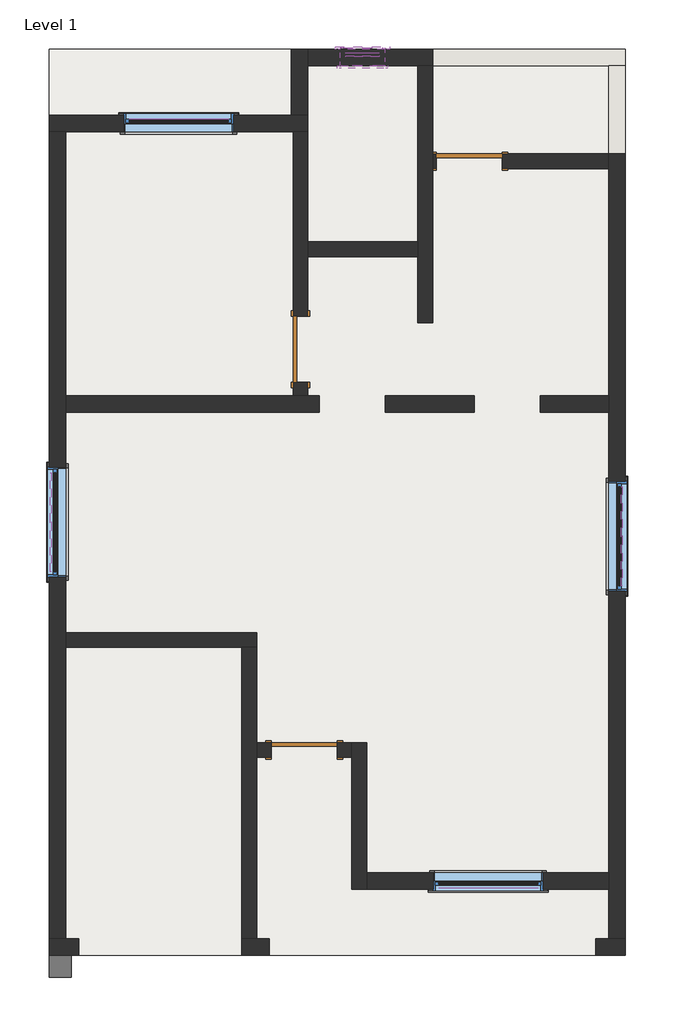
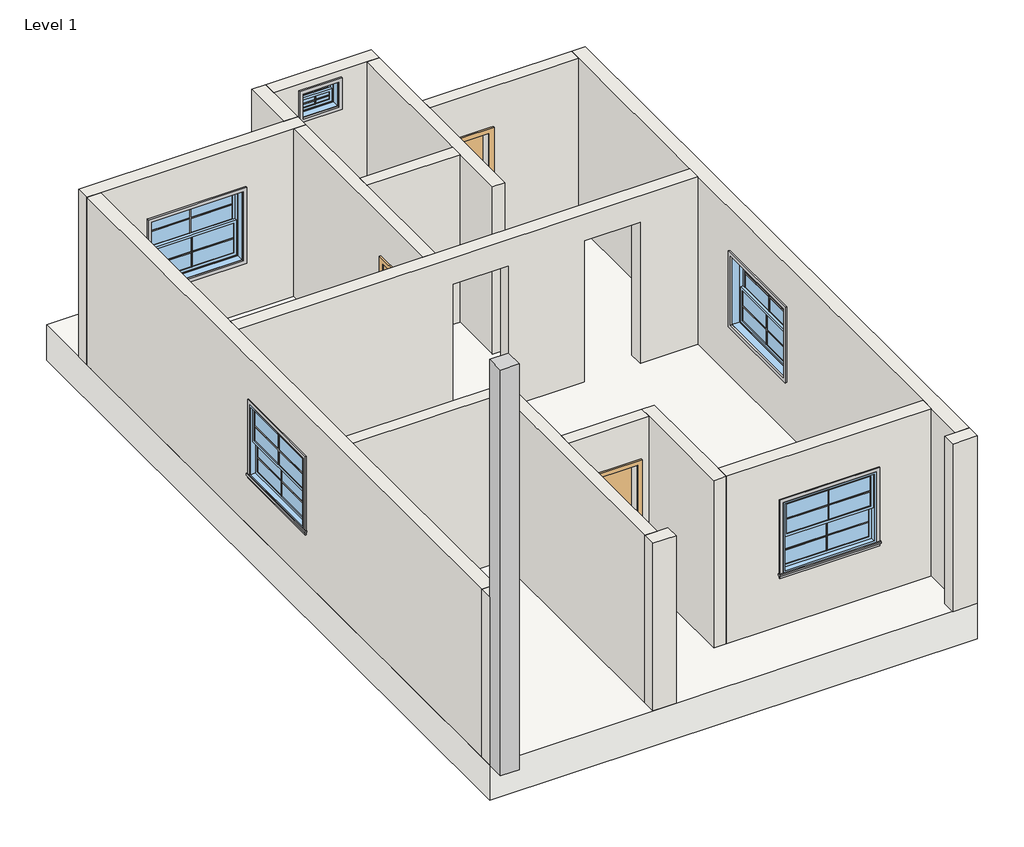
# One storey: 21 proxies, 20 walls, 5 windows, 3 doors, 1 slab.
"""IFC4 building model written with IfcOpenShell, lengths in millimetres."""

from ifc_helpers import new_model, si_unit, frame, origin, origin_with_axes, place, context, project, spatial, polyline, outline, extrude, faceted_brep, transform, mapped, element, save
from components import generic_models_2_generic_models_2_628e6232, muntin_pattern_2x2_muntin_pattern_2x2_c001a7f4, muntin_pattern_2x2_muntin_pattern_2x2_019d64ce, trim_window_exterior_flat_with_sill_7631c5ba, trim_window_exterior_flat_with_sill_f6d2a3b8, trim_window_interior_flat_picture_frame_0f2e31f9, trim_window_interior_flat_picture_frame_f985c0ae, door_719f80de, window_42222e0e, window_a144fa31

model = new_model("IFC4")

# Units and contexts
model_context = context("Model", 3, world=origin())
ifc_project = project(units=[si_unit("LENGTHUNIT", "METRE", prefix="MILLI")], contexts=[model_context])

# Site, building, storey
site = spatial("IfcSite", under=ifc_project)
building = spatial("IfcBuilding", under=site)
storey = spatial("IfcBuildingStorey", under=building, Name="Level 1", Elevation=0.0)

# Proxies
placement = place(None, origin())
generic_models_2_generic_models_2_shape = generic_models_2_generic_models_2_628e6232(model_context)
element("IfcBuildingElementProxy", 1, Name="Generic Models 2 : Generic Models 2", ObjectType="Generic Models 2 : Generic Models 2", at=placement, inside=storey, context=model_context, shape_type="MappedRepresentation", body=[
    mapped(generic_models_2_generic_models_2_shape, transform((0.0, 0.0, 0.0), x_axis=(1.0, 0.0, 0.0), y_axis=(0.0, 1.0, 0.0), z_axis=(0.0, 0.0, 1.0))),
])
muntin_pattern_2x2_muntin_pattern_2x2_shape = muntin_pattern_2x2_muntin_pattern_2x2_c001a7f4(model_context)
element("IfcBuildingElementProxy", 2, Name="Muntin Pattern_2x2 : Muntin Pattern_2x2", ObjectType="Muntin Pattern_2x2 : Muntin Pattern_2x2", at=placement, inside=storey, context=model_context, shape_type="MappedRepresentation", body=[
    mapped(muntin_pattern_2x2_muntin_pattern_2x2_shape, transform((-2405.2019453, 4921.3694012, 1546.225), x_axis=(-1.0, 0.0, 0.0), y_axis=(0.0, -1.0, 0.0), z_axis=(0.0, 0.0, 1.0))),
])
element("IfcBuildingElementProxy", 3, Name="Muntin Pattern_2x2 : Muntin Pattern_2x2", ObjectType="Muntin Pattern_2x2 : Muntin Pattern_2x2", at=placement, inside=storey, context=model_context, shape_type="MappedRepresentation", body=[
    mapped(muntin_pattern_2x2_muntin_pattern_2x2_shape, transform((-2405.2019453, 4965.8194012, 990.6), x_axis=(-1.0, 0.0, 0.0), y_axis=(0.0, -1.0, 0.0), z_axis=(0.0, 0.0, 1.0))),
])
element("IfcBuildingElementProxy", 4, Name="Muntin Pattern_2x2 : Muntin Pattern_2x2", ObjectType="Muntin Pattern_2x2 : Muntin Pattern_2x2", at=placement, inside=storey, context=model_context, shape_type="MappedRepresentation", body=[
    mapped(muntin_pattern_2x2_muntin_pattern_2x2_shape, transform((-8447.2269453, 9972.7944012, 1546.225), x_axis=(0.0, 1.0, 0.0), y_axis=(-1.0, 0.0, 0.0), z_axis=(0.0, 0.0, 1.0))),
])
element("IfcBuildingElementProxy", 5, Name="Muntin Pattern_2x2 : Muntin Pattern_2x2", ObjectType="Muntin Pattern_2x2 : Muntin Pattern_2x2", at=placement, inside=storey, context=model_context, shape_type="MappedRepresentation", body=[
    mapped(muntin_pattern_2x2_muntin_pattern_2x2_shape, transform((-8402.7769453, 9972.7944012, 990.6), x_axis=(0.0, 1.0, 0.0), y_axis=(-1.0, 0.0, 0.0), z_axis=(0.0, 0.0, 1.0))),
])
element("IfcBuildingElementProxy", 6, Name="Muntin Pattern_2x2 : Muntin Pattern_2x2", ObjectType="Muntin Pattern_2x2 : Muntin Pattern_2x2", at=placement, inside=storey, context=model_context, shape_type="MappedRepresentation", body=[
    mapped(muntin_pattern_2x2_muntin_pattern_2x2_shape, transform((-541.4769453, 9775.9444012, 1546.225), x_axis=(0.0, -1.0, 0.0), y_axis=(1.0, 0.0, 0.0), z_axis=(0.0, 0.0, 1.0))),
])
element("IfcBuildingElementProxy", 7, Name="Muntin Pattern_2x2 : Muntin Pattern_2x2", ObjectType="Muntin Pattern_2x2 : Muntin Pattern_2x2", at=placement, inside=storey, context=model_context, shape_type="MappedRepresentation", body=[
    mapped(muntin_pattern_2x2_muntin_pattern_2x2_shape, transform((-585.9269453, 9775.9444012, 990.6), x_axis=(0.0, -1.0, 0.0), y_axis=(1.0, 0.0, 0.0), z_axis=(0.0, 0.0, 1.0))),
])
element("IfcBuildingElementProxy", 8, Name="Muntin Pattern_2x2 : Muntin Pattern_2x2", ObjectType="Muntin Pattern_2x2 : Muntin Pattern_2x2", at=placement, inside=storey, context=model_context, shape_type="MappedRepresentation", body=[
    mapped(muntin_pattern_2x2_muntin_pattern_2x2_shape, transform((-6691.4519453, 15570.3194012, 1546.225), x_axis=(1.0, 0.0, 0.0), y_axis=(0.0, 1.0, 0.0), z_axis=(0.0, 0.0, 1.0))),
])
element("IfcBuildingElementProxy", 9, Name="Muntin Pattern_2x2 : Muntin Pattern_2x2", ObjectType="Muntin Pattern_2x2 : Muntin Pattern_2x2", at=placement, inside=storey, context=model_context, shape_type="MappedRepresentation", body=[
    mapped(muntin_pattern_2x2_muntin_pattern_2x2_shape, transform((-6691.4519453, 15525.8694012, 990.6), x_axis=(1.0, 0.0, 0.0), y_axis=(0.0, 1.0, 0.0), z_axis=(0.0, 0.0, 1.0))),
])
muntin_pattern_2x2_muntin_pattern_2x2_2_shape = muntin_pattern_2x2_muntin_pattern_2x2_019d64ce(model_context)
element("IfcBuildingElementProxy", 10, Name="Muntin Pattern_2x2 : Muntin Pattern_2x2", ObjectType="Muntin Pattern_2x2 : Muntin Pattern_2x2", at=placement, inside=storey, context=model_context, shape_type="MappedRepresentation", body=[
    mapped(muntin_pattern_2x2_muntin_pattern_2x2_2_shape, transform((-4145.1019453, 16484.7194012, 2536.825), x_axis=(1.0, 0.0, 0.0), y_axis=(0.0, 1.0, 0.0), z_axis=(0.0, 0.0, 1.0))),
])
element("IfcBuildingElementProxy", 11, Name="Muntin Pattern_2x2 : Muntin Pattern_2x2", ObjectType="Muntin Pattern_2x2 : Muntin Pattern_2x2", at=placement, inside=storey, context=model_context, shape_type="MappedRepresentation", body=[
    mapped(muntin_pattern_2x2_muntin_pattern_2x2_2_shape, transform((-4145.1019453, 16440.2694012, 2362.2), x_axis=(1.0, 0.0, 0.0), y_axis=(0.0, 1.0, 0.0), z_axis=(0.0, 0.0, 1.0))),
])
trim_window_exterior_flat_with_sill_shape = trim_window_exterior_flat_with_sill_7631c5ba(model_context)
element("IfcBuildingElementProxy", 12, Name="Trim-Window-Exterior-Flat : with Sill", ObjectType="Trim-Window-Exterior-Flat : with Sill", at=placement, inside=storey, context=model_context, shape_type="MappedRepresentation", body=[
    mapped(trim_window_exterior_flat_with_sill_shape, transform((-2405.2019453, 4886.4444012, 2133.6), x_axis=(1.0, 0.0, 0.0), y_axis=(0.0, 0.0, 1.0), z_axis=(0.0, -1.0, 0.0))),
])
element("IfcBuildingElementProxy", 13, Name="Trim-Window-Exterior-Flat : with Sill", ObjectType="Trim-Window-Exterior-Flat : with Sill", at=placement, inside=storey, context=model_context, shape_type="MappedRepresentation", body=[
    mapped(trim_window_exterior_flat_with_sill_shape, transform((-8482.1519453, 9972.7944012, 2133.6), x_axis=(0.0, -1.0, 0.0), y_axis=(0.0, 0.0, 1.0), z_axis=(-1.0, 0.0, 0.0))),
])
element("IfcBuildingElementProxy", 14, Name="Trim-Window-Exterior-Flat : with Sill", ObjectType="Trim-Window-Exterior-Flat : with Sill", at=placement, inside=storey, context=model_context, shape_type="MappedRepresentation", body=[
    mapped(trim_window_exterior_flat_with_sill_shape, transform((-506.5519453, 9775.9444012, 2133.6), x_axis=(0.0, 1.0, 0.0), y_axis=(0.0, 0.0, 1.0), z_axis=(1.0, 0.0, 0.0))),
])
element("IfcBuildingElementProxy", 15, Name="Trim-Window-Exterior-Flat : with Sill", ObjectType="Trim-Window-Exterior-Flat : with Sill", at=placement, inside=storey, context=model_context, shape_type="MappedRepresentation", body=[
    mapped(trim_window_exterior_flat_with_sill_shape, transform((-6691.4519453, 15605.2444012, 2133.6), x_axis=(-1.0, 0.0, 0.0), y_axis=(0.0, 0.0, 1.0), z_axis=(0.0, 1.0, 0.0))),
])
trim_window_exterior_flat_with_sill_2_shape = trim_window_exterior_flat_with_sill_f6d2a3b8(model_context)
element("IfcBuildingElementProxy", 16, Name="Trim-Window-Exterior-Flat : with Sill", ObjectType="Trim-Window-Exterior-Flat : with Sill", at=placement, inside=storey, context=model_context, shape_type="MappedRepresentation", body=[
    mapped(trim_window_exterior_flat_with_sill_2_shape, transform((-4145.1019453, 16519.6444012, 2743.2), x_axis=(-1.0, 0.0, 0.0), y_axis=(0.0, 0.0, 1.0), z_axis=(0.0, 1.0, 0.0))),
])
trim_window_interior_flat_picture_frame_shape = trim_window_interior_flat_picture_frame_0f2e31f9(model_context)
element("IfcBuildingElementProxy", 17, Name="Trim-Window-Interior-Flat : Picture Frame", ObjectType="Trim-Window-Interior-Flat : Picture Frame", at=placement, inside=storey, context=model_context, shape_type="MappedRepresentation", body=[
    mapped(trim_window_interior_flat_picture_frame_shape, transform((-2405.2019453, 5115.0444012, 2133.6), x_axis=(-1.0, 0.0, 0.0), y_axis=(0.0, 0.0, 1.0), z_axis=(0.0, 1.0, 0.0))),
])
element("IfcBuildingElementProxy", 18, Name="Trim-Window-Interior-Flat : Picture Frame", ObjectType="Trim-Window-Interior-Flat : Picture Frame", at=placement, inside=storey, context=model_context, shape_type="MappedRepresentation", body=[
    mapped(trim_window_interior_flat_picture_frame_shape, transform((-8253.5519453, 9972.7944012, 2133.6), x_axis=(0.0, 1.0, 0.0), y_axis=(0.0, 0.0, 1.0), z_axis=(1.0, 0.0, 0.0))),
])
element("IfcBuildingElementProxy", 19, Name="Trim-Window-Interior-Flat : Picture Frame", ObjectType="Trim-Window-Interior-Flat : Picture Frame", at=placement, inside=storey, context=model_context, shape_type="MappedRepresentation", body=[
    mapped(trim_window_interior_flat_picture_frame_shape, transform((-735.1519453, 9775.9444012, 2133.6), x_axis=(0.0, -1.0, 0.0), y_axis=(0.0, 0.0, 1.0), z_axis=(-1.0, 0.0, 0.0))),
])
element("IfcBuildingElementProxy", 20, Name="Trim-Window-Interior-Flat : Picture Frame", ObjectType="Trim-Window-Interior-Flat : Picture Frame", at=placement, inside=storey, context=model_context, shape_type="MappedRepresentation", body=[
    mapped(trim_window_interior_flat_picture_frame_shape, transform((-6691.4519453, 15376.6444012, 2133.6), x_axis=(1.0, 0.0, 0.0), y_axis=(0.0, 0.0, 1.0), z_axis=(0.0, -1.0, 0.0))),
])
trim_window_interior_flat_picture_frame_2_shape = trim_window_interior_flat_picture_frame_f985c0ae(model_context)
element("IfcBuildingElementProxy", 21, Name="Trim-Window-Interior-Flat : Picture Frame", ObjectType="Trim-Window-Interior-Flat : Picture Frame", at=placement, inside=storey, context=model_context, shape_type="MappedRepresentation", body=[
    mapped(trim_window_interior_flat_picture_frame_2_shape, transform((-4145.1019453, 16291.0444012, 2743.2), x_axis=(1.0, 0.0, 0.0), y_axis=(0.0, 0.0, 1.0), z_axis=(0.0, -1.0, 0.0))),
])

# Doors
door_shape = door_719f80de(model_context)
element("IfcDoor", 22, ObjectType="Single-Flush : 36\" x 84\"", at=placement, inside=storey, context=model_context, shape_type="MappedRepresentation", body=[
    mapped(door_shape, transform((-4951.5519453, 6816.8444012, 0.0), x_axis=(-1.0, 0.0, 0.0), y_axis=(0.0, -1.0, 0.0), z_axis=(0.0, 0.0, 1.0))),
])
element("IfcDoor", 23, ObjectType="Single-Flush : 36\" x 84\"", at=placement, inside=storey, context=model_context, shape_type="MappedRepresentation", body=[
    mapped(door_shape, transform((-5002.3519453, 12366.7444012, 0.0), x_axis=(0.0, -1.0, 0.0), y_axis=(1.0, 0.0, 0.0), z_axis=(0.0, 0.0, 1.0))),
])
element("IfcDoor", 24, ObjectType="Single-Flush : 36\" x 84\"", at=placement, inside=storey, context=model_context, shape_type="MappedRepresentation", body=[
    mapped(door_shape, transform((-2665.5519453, 14970.2444012, 0.0), x_axis=(-1.0, 0.0, 0.0), y_axis=(0.0, -1.0, 0.0), z_axis=(0.0, 0.0, 1.0))),
])

# Slab
element("IfcSlab", 25, ObjectType="FLOOR 2'", at=placement, inside=storey, context=model_context, shape_type="SweptSolid", body=[
    extrude(outline(polyline([(-506.5519453, 16519.6444012), (-506.5519453, 3972.0444012), (-8482.1519453, 3972.0444012), (-8482.1519453, 16519.6444012), (-506.5519453, 16519.6444012)])), frame((0.0, 0.0, -609.6), z_axis=(0.0, 0.0, 1.0), x_axis=(1.0, 0.0, 0.0)), (0.0, 0.0, 1.0), 609.6),
])

# Walls
element("IfcWall", 26, ObjectType="WALL 6\"", at=placement, inside=storey, context=model_context, shape_type="Brep", body=[
    faceted_brep([(-3376.7519453, 16291.0444012, 2895.6), (-3376.7519453, 16291.0444012, 0.0), (-3376.7519453, 13852.6444012, 0.0), (-3376.7519453, 13649.4444012, 0.0), (-3376.7519453, 12735.0444012, 0.0), (-3376.7519453, 12735.0444012, 2895.6), (-3376.7519453, 13649.4444012, 2895.6), (-3376.7519453, 13852.6444012, 2895.6), (-3173.5519453, 16291.0444012, 0.0), (-3173.5519453, 16291.0444012, 2895.6), (-3173.5519453, 15071.8444012, 2895.6), (-3173.5519453, 14868.6444012, 2895.6), (-3173.5519453, 12735.0444012, 2895.6), (-3173.5519453, 12735.0444012, 0.0), (-3173.5519453, 14868.6444012, 0.0), (-3173.5519453, 15071.8444012, 0.0)], [[[0, 1, 2, 3, 4, 5, 6, 7]], [[8, 9, 10, 11, 12, 13, 14, 15]], [[4, 3, 2, 1, 8, 15, 14, 13]], [[5, 4, 13, 12]], [[0, 9, 8, 1]], [[0, 7, 6, 5, 12, 11, 10, 9]]]),
])
element("IfcWall", 27, ObjectType="WALL 6\"", at=placement, inside=storey, context=model_context, shape_type="SweptSolid", body=[
    extrude(outline(polyline([(0.0, -3173.5519453), (0.0, -3122.7519453), (2133.6, -3122.7519453), (2133.6, -2208.3519453), (0.0, -2208.3519453), (0.0, -735.1519453), (2895.6, -735.1519453), (2895.6, -3173.5519453), (0.0, -3173.5519453)])), frame((0.0, 14868.6444012, 0.0), z_axis=(0.0, 1.0, 0.0), x_axis=(0.0, 0.0, 1.0)), (0.0, 0.0, 1.0), 203.2),
])
element("IfcWall", 28, ObjectType="WALL 6\"", at=placement, inside=storey, context=model_context, shape_type="Brep", body=[
    faceted_brep([(-5103.9519453, 11909.5444012, 2133.6), (-5103.9519453, 11909.5444012, 0.0), (-5103.9519453, 11719.0444012, 0.0), (-5103.9519453, 11719.0444012, 2895.6), (-5103.9519453, 15376.6444012, 2895.6), (-5103.9519453, 15376.6444012, 0.0), (-5103.9519453, 12823.9444012, 0.0), (-5103.9519453, 12823.9444012, 2133.6), (-4900.7519453, 11719.0444012, 0.0), (-4900.7519453, 11909.5444012, 0.0), (-4900.7519453, 11909.5444012, 2133.6), (-4900.7519453, 12823.9444012, 2133.6), (-4900.7519453, 12823.9444012, 0.0), (-4900.7519453, 13649.4444012, 0.0), (-4900.7519453, 13852.6444012, 0.0), (-4900.7519453, 15376.6444012, 0.0), (-4900.7519453, 15376.6444012, 2895.6), (-4900.7519453, 13852.6444012, 2895.6), (-4900.7519453, 13649.4444012, 2895.6), (-4900.7519453, 11719.0444012, 2895.6)], [[[0, 1, 2, 3, 4, 5, 6, 7]], [[8, 9, 10, 11, 12, 13, 14, 15, 16, 17, 18, 19]], [[6, 5, 15, 14, 13, 12]], [[2, 1, 9, 8]], [[5, 4, 16, 15]], [[3, 2, 8, 19]], [[10, 9, 1, 0]], [[11, 10, 0, 7]], [[12, 11, 7, 6]], [[4, 3, 19, 18, 17, 16]]]),
])
element("IfcWall", 29, ObjectType="WALL 6\"", at=placement, inside=storey, context=model_context, shape_type="SweptSolid", body=[
    extrude(outline(polyline([(-3376.7519453, 13649.4444012), (-4900.7519453, 13649.4444012), (-4900.7519453, 13852.6444012), (-3376.7519453, 13852.6444012), (-3376.7519453, 13649.4444012)])), origin_with_axes(), (0.0, 0.0, 1.0), 2895.6),
])
element("IfcWall", 30, ObjectType="WALL 6\"", at=placement, inside=storey, context=model_context, shape_type="Brep", body=[
    faceted_brep([(-8253.5519453, 8239.2444012, 0.0), (-5815.1519453, 8239.2444012, 0.0), (-5611.9519453, 8239.2444012, 0.0), (-5611.9519453, 8239.2444012, 2895.6), (-5815.1519453, 8239.2444012, 2895.6), (-8253.5519453, 8239.2444012, 2895.6), (-8253.5519453, 8442.4444012, 0.0), (-8253.5519453, 8442.4444012, 2895.6), (-5611.9519453, 8442.4444012, 2895.6), (-5611.9519453, 8442.4444012, 0.0)], [[[0, 1, 2, 3, 4, 5]], [[6, 7, 8, 9]], [[2, 1, 0, 6, 9]], [[0, 5, 7, 6]], [[3, 2, 9, 8]], [[5, 4, 3, 8, 7]]]),
])
element("IfcWall", 31, ObjectType="WALL 6\"", at=placement, inside=storey, context=model_context, shape_type="Brep", body=[
    faceted_brep([(-5815.1519453, 8239.2444012, 0.0), (-5815.1519453, 4200.6444012, 0.0), (-5815.1519453, 4200.6444012, 2895.6), (-5815.1519453, 8239.2444012, 2895.6), (-5611.9519453, 8239.2444012, 0.0), (-5611.9519453, 8239.2444012, 2895.6), (-5611.9519453, 6918.4444012, 2895.6), (-5611.9519453, 6715.2444012, 2895.6), (-5611.9519453, 4200.6444012, 2895.6), (-5611.9519453, 4200.6444012, 0.0), (-5611.9519453, 6715.2444012, 0.0), (-5611.9519453, 6918.4444012, 0.0)], [[[0, 1, 2, 3]], [[4, 5, 6, 7, 8, 9, 10, 11]], [[1, 0, 4, 11, 10, 9]], [[0, 3, 5, 4]], [[2, 1, 9, 8]], [[3, 2, 8, 7, 6, 5]]]),
])
element("IfcWall", 32, ObjectType="WALL 6\"", at=placement, inside=storey, context=model_context, shape_type="Brep", body=[
    faceted_brep([(-4291.1519453, 6918.4444012, 0.0), (-4291.1519453, 6715.2444012, 0.0), (-4291.1519453, 4886.4444012, 0.0), (-4291.1519453, 4886.4444012, 2895.6), (-4291.1519453, 6715.2444012, 2895.6), (-4291.1519453, 6918.4444012, 2895.6), (-4087.9519453, 6918.4444012, 0.0), (-4087.9519453, 6918.4444012, 2895.6), (-4087.9519453, 5115.0444012, 2895.6), (-4087.9519453, 4886.4444012, 2895.6), (-4087.9519453, 4886.4444012, 0.0), (-4087.9519453, 5115.0444012, 0.0)], [[[0, 1, 2, 3, 4, 5]], [[6, 7, 8, 9, 10, 11]], [[2, 1, 0, 6, 11, 10]], [[3, 2, 10, 9]], [[0, 5, 7, 6]], [[5, 4, 3, 9, 8, 7]]]),
])
element("IfcWall", 33, ObjectType="WALL 6\"", at=placement, inside=storey, context=model_context, shape_type="SweptSolid", body=[
    extrude(outline(polyline([(0.0, -5611.9519453), (0.0, -5408.7519453), (2133.6, -5408.7519453), (2133.6, -4494.3519453), (0.0, -4494.3519453), (0.0, -4291.1519453), (2895.6, -4291.1519453), (2895.6, -5611.9519453), (0.0, -5611.9519453)])), frame((0.0, 6715.2444012, 0.0), z_axis=(0.0, 1.0, 0.0), x_axis=(0.0, 0.0, 1.0)), (0.0, 0.0, 1.0), 203.2),
])
element("IfcWall", 34, ObjectType="WALL 9\"", at=placement, inside=storey, context=model_context, shape_type="Brep", body=[
    faceted_brep([(-8482.1519453, 15376.6444012, 0.0), (-8253.5519453, 15376.6444012, 0.0), (-5103.9519453, 15376.6444012, 0.0), (-4900.7519453, 15376.6444012, 0.0), (-4900.7519453, 15376.6444012, 2895.6), (-5103.9519453, 15376.6444012, 2895.6), (-8253.5519453, 15376.6444012, 2895.6), (-8482.1519453, 15376.6444012, 2895.6), (-7453.4519453, 15376.6444012, 2133.6), (-5929.4519453, 15376.6444012, 2133.6), (-5929.4519453, 15376.6444012, 914.4), (-7453.4519453, 15376.6444012, 914.4), (-8482.1519453, 15605.2444012, 0.0), (-8482.1519453, 15605.2444012, 2895.6), (-5129.3519453, 15605.2444012, 2895.6), (-4900.7519453, 15605.2444012, 2895.6), (-4900.7519453, 15605.2444012, 0.0), (-5129.3519453, 15605.2444012, 0.0), (-7453.4519453, 15605.2444012, 2133.6), (-7453.4519453, 15605.2444012, 914.4), (-5929.4519453, 15605.2444012, 914.4), (-5929.4519453, 15605.2444012, 2133.6)], [[[0, 1, 2, 3, 4, 5, 6, 7], [8, 9, 10, 11]], [[12, 13, 14, 15, 16, 17], [18, 19, 20, 21]], [[3, 2, 1, 0, 12, 17, 16]], [[4, 3, 16, 15]], [[0, 7, 13, 12]], [[19, 18, 8, 11]], [[20, 19, 11, 10]], [[21, 20, 10, 9]], [[18, 21, 9, 8]], [[7, 6, 5, 4, 15, 14, 13]]]),
])
element("IfcWall", 35, ObjectType="WALL 9\"", at=placement, inside=storey, context=model_context, shape_type="Brep", body=[
    faceted_brep([(-4900.7519453, 15605.2444012, 0.0), (-4900.7519453, 16291.0444012, 0.0), (-4900.7519453, 16519.6444012, 0.0), (-4900.7519453, 16519.6444012, 2895.6), (-4900.7519453, 16291.0444012, 2895.6), (-4900.7519453, 15605.2444012, 2895.6), (-5129.3519453, 15605.2444012, 0.0), (-5129.3519453, 15605.2444012, 2895.6), (-5129.3519453, 16519.6444012, 2895.6), (-5129.3519453, 16519.6444012, 0.0)], [[[0, 1, 2, 3, 4, 5]], [[6, 7, 8, 9]], [[2, 1, 0, 6, 9]], [[0, 5, 7, 6]], [[3, 2, 9, 8]], [[5, 4, 3, 8, 7]]]),
])
element("IfcWall", 36, ObjectType="WALL 9\"", at=placement, inside=storey, context=model_context, shape_type="Brep", body=[
    faceted_brep([(-4900.7519453, 16291.0444012, 0.0), (-3376.7519453, 16291.0444012, 0.0), (-3173.5519453, 16291.0444012, 0.0), (-3173.5519453, 16291.0444012, 914.4), (-3173.5519453, 16291.0444012, 2895.6), (-3376.7519453, 16291.0444012, 2895.6), (-4900.7519453, 16291.0444012, 2895.6), (-4449.9019453, 16291.0444012, 2743.2), (-3840.3019453, 16291.0444012, 2743.2), (-3840.3019453, 16291.0444012, 2286.0), (-4449.9019453, 16291.0444012, 2286.0), (-4900.7519453, 16519.6444012, 0.0), (-4900.7519453, 16519.6444012, 2895.6), (-3173.5519453, 16519.6444012, 2895.6), (-3173.5519453, 16519.6444012, 914.4), (-3173.5519453, 16519.6444012, 0.0), (-4449.9019453, 16519.6444012, 2743.2), (-4449.9019453, 16519.6444012, 2286.0), (-3840.3019453, 16519.6444012, 2286.0), (-3840.3019453, 16519.6444012, 2743.2)], [[[0, 1, 2, 3, 4, 5, 6], [7, 8, 9, 10]], [[11, 12, 13, 14, 15], [16, 17, 18, 19]], [[2, 1, 0, 11, 15]], [[0, 6, 12, 11]], [[17, 16, 7, 10]], [[18, 17, 10, 9]], [[19, 18, 9, 8]], [[16, 19, 8, 7]], [[2, 15, 14, 13, 4, 3]], [[6, 5, 4, 13, 12]]]),
])
element("IfcWall", 37, ObjectType="WALL 9\"", at=placement, inside=storey, context=model_context, shape_type="Brep", body=[
    faceted_brep([(-735.1519453, 15071.8444012, 2895.6), (-735.1519453, 15071.8444012, 914.4), (-735.1519453, 15071.8444012, 0.0), (-735.1519453, 14868.6444012, 0.0), (-735.1519453, 11719.0444012, 0.0), (-735.1519453, 11490.4444012, 0.0), (-735.1519453, 5115.0444012, 0.0), (-735.1519453, 4886.4444012, 0.0), (-735.1519453, 4200.6444012, 0.0), (-735.1519453, 4200.6444012, 2895.6), (-735.1519453, 4886.4444012, 2895.6), (-735.1519453, 5115.0444012, 2895.6), (-735.1519453, 11490.4444012, 2895.6), (-735.1519453, 11719.0444012, 2895.6), (-735.1519453, 14868.6444012, 2895.6), (-735.1519453, 10537.9444012, 2133.6), (-735.1519453, 9013.9444012, 2133.6), (-735.1519453, 9013.9444012, 914.4), (-735.1519453, 10537.9444012, 914.4), (-506.5519453, 15071.8444012, 0.0), (-506.5519453, 15071.8444012, 914.4), (-506.5519453, 15071.8444012, 2895.6), (-506.5519453, 4200.6444012, 2895.6), (-506.5519453, 4200.6444012, 0.0), (-506.5519453, 10537.9444012, 2133.6), (-506.5519453, 10537.9444012, 914.4), (-506.5519453, 9013.9444012, 914.4), (-506.5519453, 9013.9444012, 2133.6)], [[[0, 1, 2, 3, 4, 5, 6, 7, 8, 9, 10, 11, 12, 13, 14], [15, 16, 17, 18]], [[19, 20, 21, 22, 23], [24, 25, 26, 27]], [[8, 7, 6, 5, 4, 3, 2, 19, 23]], [[9, 8, 23, 22]], [[25, 24, 15, 18]], [[26, 25, 18, 17]], [[27, 26, 17, 16]], [[24, 27, 16, 15]], [[0, 21, 20, 19, 2, 1]], [[0, 14, 13, 12, 11, 10, 9, 22, 21]]]),
])
element("IfcWall", 38, ObjectType="WALL 9\"", at=placement, inside=storey, context=model_context, shape_type="Brep", body=[
    faceted_brep([(-8482.1519453, 15376.6444012, 0.0), (-8482.1519453, 4200.6444012, 0.0), (-8482.1519453, 4200.6444012, 2895.6), (-8482.1519453, 15376.6444012, 2895.6), (-8482.1519453, 9210.7944012, 2133.6), (-8482.1519453, 9210.7944012, 914.4), (-8482.1519453, 10734.7944012, 914.4), (-8482.1519453, 10734.7944012, 2133.6), (-8253.5519453, 15376.6444012, 0.0), (-8253.5519453, 15376.6444012, 2895.6), (-8253.5519453, 11719.0444012, 2895.6), (-8253.5519453, 11490.4444012, 2895.6), (-8253.5519453, 8442.4444012, 2895.6), (-8253.5519453, 8239.2444012, 2895.6), (-8253.5519453, 4200.6444012, 2895.6), (-8253.5519453, 4200.6444012, 0.0), (-8253.5519453, 8239.2444012, 0.0), (-8253.5519453, 8442.4444012, 0.0), (-8253.5519453, 11490.4444012, 0.0), (-8253.5519453, 11719.0444012, 0.0), (-8253.5519453, 9210.7944012, 2133.6), (-8253.5519453, 10734.7944012, 2133.6), (-8253.5519453, 10734.7944012, 914.4), (-8253.5519453, 9210.7944012, 914.4)], [[[0, 1, 2, 3], [4, 5, 6, 7]], [[8, 9, 10, 11, 12, 13, 14, 15, 16, 17, 18, 19], [20, 21, 22, 23]], [[1, 0, 8, 19, 18, 17, 16, 15]], [[0, 3, 9, 8]], [[2, 1, 15, 14]], [[5, 4, 20, 23]], [[6, 5, 23, 22]], [[7, 6, 22, 21]], [[4, 7, 21, 20]], [[3, 2, 14, 13, 12, 11, 10, 9]]]),
])
element("IfcWall", 39, ObjectType="WALL 9\"", at=placement, inside=storey, context=model_context, shape_type="Brep", body=[
    faceted_brep([(-735.1519453, 11490.4444012, 0.0), (-735.1519453, 11490.4444012, 2895.6), (-8253.5519453, 11490.4444012, 2895.6), (-8253.5519453, 11490.4444012, 0.0), (-4743.1442114, 11490.4444012, 0.0), (-4743.1442114, 11490.4444012, 2438.4), (-3828.7442114, 11490.4444012, 2438.4), (-3828.7442114, 11490.4444012, 0.0), (-2596.3234852, 11490.4444012, 0.0), (-2596.3234852, 11490.4444012, 2438.4), (-1681.9234852, 11490.4444012, 2438.4), (-1681.9234852, 11490.4444012, 0.0), (-735.1519453, 11719.0444012, 2895.6), (-735.1519453, 11719.0444012, 0.0), (-1681.9234852, 11719.0444012, 0.0), (-1681.9234852, 11719.0444012, 2438.4), (-2596.3234852, 11719.0444012, 2438.4), (-2596.3234852, 11719.0444012, 0.0), (-3828.7442114, 11719.0444012, 0.0), (-3828.7442114, 11719.0444012, 2438.4), (-4743.1442114, 11719.0444012, 2438.4), (-4743.1442114, 11719.0444012, 0.0), (-4900.7519453, 11719.0444012, 0.0), (-5103.9519453, 11719.0444012, 0.0), (-8253.5519453, 11719.0444012, 0.0), (-8253.5519453, 11719.0444012, 2895.6), (-5103.9519453, 11719.0444012, 2895.6), (-4900.7519453, 11719.0444012, 2895.6)], [[[0, 1, 2, 3, 4, 5, 6, 7, 8, 9, 10, 11]], [[12, 13, 14, 15, 16, 17, 18, 19, 20, 21, 22, 23, 24, 25, 26, 27]], [[3, 24, 23, 22, 21, 4]], [[13, 0, 11, 14]], [[17, 8, 7, 18]], [[3, 2, 25, 24]], [[1, 0, 13, 12]], [[9, 16, 15, 10]], [[16, 9, 8, 17]], [[10, 15, 14, 11]], [[5, 20, 19, 6]], [[20, 5, 4, 21]], [[6, 19, 18, 7]], [[2, 1, 12, 27, 26, 25]]]),
])
element("IfcWall", 40, ObjectType="WALL 9\"", at=placement, inside=storey, context=model_context, shape_type="SweptSolid", body=[
    extrude(outline(polyline([(0.0, -4087.9519453), (0.0, -735.1519453), (2895.6, -735.1519453), (2895.6, -4087.9519453), (0.0, -4087.9519453)]), holes=[polyline([(2133.6, -1643.2019453), (914.4, -1643.2019453), (914.4, -3167.2019453), (2133.6, -3167.2019453), (2133.6, -1643.2019453)])]), frame((0.0, 4886.4444012, 0.0), z_axis=(0.0, 1.0, 0.0), x_axis=(0.0, 0.0, 1.0)), (0.0, 0.0, 1.0), 228.6),
])
element("IfcWall", 41, ObjectType="WALL 9\"", at=placement, inside=storey, context=model_context, shape_type="Brep", body=[
    faceted_brep([(-8482.1519453, 3972.0444012, 0.0), (-8075.7519453, 3972.0444012, 0.0), (-8075.7519453, 3972.0444012, 2895.6), (-8482.1519453, 3972.0444012, 2895.6), (-8482.1519453, 4200.6444012, 0.0), (-8482.1519453, 4200.6444012, 2895.6), (-8253.5519453, 4200.6444012, 2895.6), (-8075.7519453, 4200.6444012, 2895.6), (-8075.7519453, 4200.6444012, 0.0), (-8253.5519453, 4200.6444012, 0.0)], [[[0, 1, 2, 3]], [[4, 5, 6, 7, 8, 9]], [[1, 0, 4, 9, 8]], [[2, 1, 8, 7]], [[0, 3, 5, 4]], [[3, 2, 7, 6, 5]]]),
])
element("IfcWall", 42, ObjectType="WALL 9\"", at=placement, inside=storey, context=model_context, shape_type="Brep", body=[
    faceted_brep([(-5815.1519453, 3972.0444012, 0.0), (-5434.1519453, 3972.0444012, 0.0), (-5434.1519453, 3972.0444012, 2895.6), (-5815.1519453, 3972.0444012, 2895.6), (-5815.1519453, 4200.6444012, 0.0), (-5815.1519453, 4200.6444012, 2895.6), (-5611.9519453, 4200.6444012, 2895.6), (-5434.1519453, 4200.6444012, 2895.6), (-5434.1519453, 4200.6444012, 0.0), (-5611.9519453, 4200.6444012, 0.0)], [[[0, 1, 2, 3]], [[4, 5, 6, 7, 8, 9]], [[1, 0, 4, 9, 8]], [[2, 1, 8, 7]], [[0, 3, 5, 4]], [[3, 2, 7, 6, 5]]]),
])
element("IfcWall", 43, ObjectType="WALL 9\"", at=placement, inside=storey, context=model_context, shape_type="Brep", body=[
    faceted_brep([(-506.5519453, 4200.6444012, 0.0), (-735.1519453, 4200.6444012, 0.0), (-912.9519453, 4200.6444012, 0.0), (-912.9519453, 4200.6444012, 2895.6), (-735.1519453, 4200.6444012, 2895.6), (-506.5519453, 4200.6444012, 2895.6), (-506.5519453, 3972.0444012, 0.0), (-506.5519453, 3972.0444012, 2895.6), (-912.9519453, 3972.0444012, 2895.6), (-912.9519453, 3972.0444012, 0.0)], [[[0, 1, 2, 3, 4, 5]], [[6, 7, 8, 9]], [[2, 1, 0, 6, 9]], [[3, 2, 9, 8]], [[0, 5, 7, 6]], [[5, 4, 3, 8, 7]]]),
])
element("IfcWall", 44, ObjectType="WALL 9\"", at=placement, inside=storey, context=model_context, shape_type="Brep", body=[
    faceted_brep([(-3173.5519453, 16291.0444012, 0.0), (-735.1519453, 16291.0444012, 0.0), (-506.5519453, 16291.0444012, 0.0), (-506.5519453, 16291.0444012, 914.4), (-735.1519453, 16291.0444012, 914.4), (-3173.5519453, 16291.0444012, 914.4), (-3173.5519453, 16519.6444012, 0.0), (-3173.5519453, 16519.6444012, 914.4), (-506.5519453, 16519.6444012, 914.4), (-506.5519453, 16519.6444012, 0.0)], [[[0, 1, 2, 3, 4, 5]], [[6, 7, 8, 9]], [[2, 1, 0, 6, 9]], [[5, 4, 3, 8, 7]], [[0, 5, 7, 6]], [[3, 2, 9, 8]]]),
])
element("IfcWall", 45, ObjectType="WALL 9\"", at=placement, inside=storey, context=model_context, shape_type="SweptSolid", body=[
    extrude(outline(polyline([(-735.1519453, 15071.8444012), (-735.1519453, 16291.0444012), (-506.5519453, 16291.0444012), (-506.5519453, 15071.8444012), (-735.1519453, 15071.8444012)])), origin_with_axes(), (0.0, 0.0, 1.0), 914.4),
])

# Windows
window_shape = window_42222e0e(model_context)
element("IfcWindow", 46, ObjectType="Window-Double-Hung : 24\" x 1'6\"", at=placement, inside=storey, context=model_context, shape_type="MappedRepresentation", body=[
    mapped(window_shape, transform((-4145.1019453, 16405.3444012, 1371.6), x_axis=(1.0, 0.0, 0.0), y_axis=(0.0, 1.0, 0.0), z_axis=(0.0, 0.0, 1.0))),
])
window_2_shape = window_a144fa31(model_context)
element("IfcWindow", 47, ObjectType="Window-Double-Hung : 60\"X48\"", at=placement, inside=storey, context=model_context, shape_type="MappedRepresentation", body=[
    mapped(window_2_shape, transform((-2405.2019453, 5000.7444012, 0.0), x_axis=(-1.0, 0.0, 0.0), y_axis=(0.0, -1.0, 0.0), z_axis=(0.0, 0.0, 1.0))),
])
element("IfcWindow", 48, ObjectType="Window-Double-Hung : 60\"X48\"", at=placement, inside=storey, context=model_context, shape_type="MappedRepresentation", body=[
    mapped(window_2_shape, transform((-8367.8519453, 9972.7944012, 0.0), x_axis=(0.0, 1.0, 0.0), y_axis=(-1.0, 0.0, 0.0), z_axis=(0.0, 0.0, 1.0))),
])
element("IfcWindow", 49, ObjectType="Window-Double-Hung : 60\"X48\"", at=placement, inside=storey, context=model_context, shape_type="MappedRepresentation", body=[
    mapped(window_2_shape, transform((-620.8519453, 9775.9444012, 0.0), x_axis=(0.0, -1.0, 0.0), y_axis=(1.0, 0.0, 0.0), z_axis=(0.0, 0.0, 1.0))),
])
element("IfcWindow", 50, ObjectType="Window-Double-Hung : 60\"X48\"", at=placement, inside=storey, context=model_context, shape_type="MappedRepresentation", body=[
    mapped(window_2_shape, transform((-6691.4519453, 15490.9444012, 0.0), x_axis=(1.0, 0.0, 0.0), y_axis=(0.0, 1.0, 0.0), z_axis=(0.0, 0.0, 1.0))),
])

save(model, "model.ifc")

# Revit data of these elements
# Type "Muntin Pattern_2x2 : Muntin Pattern_2x2"
#   Width [instance default] = 4' - 0"
#   Thickness = 0' - 0 1/2"
#   Height [instance default] = 4' - 0"
#   Distance = 0' - 0 3/4"
#   Interior Material [instance default] = none
#   Exterior Material [instance default] = none
#   Default Elevation = 0
# Type "Trim-Window-Exterior-Flat : with Sill"
#   Trim Width = 0' - 2 1/4"
#   Trim Thickness_Picture Frame = 0' - 1 1/4"
#   Trim Thickness_with Sill = 0' - 0 3/4"
#   Sill Thickness = 0' - 1 1/4"
#   Opening Width [instance default] = 2' - 0"
#   Opening Height [instance default] = 3' - 0"
#   Default Elevation = 4' - 0"
#   Sill = yes
#   Picture Frame = no
#   Trim Material [instance default] = none
# Type "Trim-Window-Interior-Flat : Picture Frame"
#   Trim Thickness_Picture Frame = 0' - 1 1/4"
#   Trim Width = 0' - 2 1/4"
#   Trim Thickness_with Sill = 0' - 0 3/4"
#   Sill Thickness = 0' - 1 1/4"
#   Opening Width [instance default] = 2' - 0"
#   Opening Height [instance default] = 3' - 0"
#   Default Elevation = 4' - 0"
#   Sill = no
#   Picture Frame = yes
#   Trim Material [instance default] = none
# Type "Single-Flush : 36\" x 84\""
#   Type Mark = "1"
#   Construction Type Id = "MDOOR"
#   Assembly Code = "C1020"
#   Analytic Construction = "Metal"
#   Thickness = 0' - 2"
#   Heat Transfer Coefficient (U) = 0.651978 BTU/(h·ft²·°F)
#   Height = 7' - 0"
#   Trim Projection Ext = 0' - 1"
#   Trim Projection Int = 0' - 1"
#   Trim Width = 0' - 3"
#   Width = 3' - 0"
#   Define Thermal Properties by = 1
#   Define Thermal Properties by = 1
#   Door Material = Door - Panel
#   Frame Material = Door - Frame
#   Visual Light Transmittance = 0
#   Solar Heat Gain Coefficient = 0
#   Function = (empty or 0)
#   Wall Closure = (empty or 0)
# Type "FLOOR 2'"
#   Assembly Code = "B1010"
#   Function = 0
#   Layers, outside or top first: 2' - 0" no material (function 1)
# Type "WALL 6\""
#   Assembly Code = "B2010"
#   Layers, outside or top first: 0' - 8" no material (function 1)
# Type "WALL 9\""
#   Assembly Code = "B2010"
#   Layers, outside or top first: 0' - 9" no material (function 1)
# Type "Window-Double-Hung : 24\" x 1'6\""
#   Type Mark = "19"
#   Fire Rating = "0.5h"
#   Construction Type Id = "DG-DR"
#   Assembly Code = "B2020100"
#   Analytic Construction = "Double glazing - domestic"
#   Wall Thickness [instance default] = 0' - 6"
#   Window Inset [instance default] = 0' - 0"
#   Visual Light Transmittance = 0.81
#   Thermal Resistance (R) = 1.8146 (h·ft²·°F)/BTU
#   Solar Heat Gain Coefficient = 0.76
#   Muntin Width = 1' - 6"
#   Muntin Height = 0' - 5 1/8"
#   Interior Wall Closure [instance default] = 0' - 1 1/2"
#   Rough Width = 2' - 0 1/2"
#   Rough Height = 1' - 6 1/2"
#   Frame Extension [instance default] = 0' - 1 1/4"
#   Exterior Wall Closure [instance default] = 0' - 0 1/2"
#   Extension Jamb [instance default] = 0' - 1 1/2"
#   Heat Transfer Coefficient (U) = 0.5511 BTU/(h·ft²·°F)
#   Height = 1' - 6"
#   Width = 2' - 0"
#   Top Muntin Visibility = yes
#   Indicator Visibility [instance default] = yes
#   Extension Jamb Visibility [instance default] = yes
#   Interior Trim Visibility [instance default] = yes
#   Exterior Trim Visibility [instance default] = yes
#   Define Thermal Properties by = 1
#   Bottom Muntin Visibility = yes
#   Muntin Pattern = Muntin Pattern_2x2 : Muntin Pattern_2x2
#   Interior Trim Material = Wood - Stained
#   Interior Trim = Trim-Window-Interior-Flat : Picture Frame
#   Exterior Trim Material = Clad - White
#   Exterior Trim = Trim-Window-Exterior-Flat : with Sill
#   Glass Panel Material = Glass
#   Exterior Frame Material = Clad - White
#   Interior Frame Material = Wood - Stained
#   Wall Closure = (empty or 0)
# Type "Window-Double-Hung : 60\"X48\""
#   Type Mark = "18"
#   Fire Rating = "0.5h"
#   Construction Type Id = "DG-DR"
#   Assembly Code = "B2020100"
#   Analytic Construction = "Double glazing - domestic"
#   Wall Thickness [instance default] = 0' - 6"
#   Window Inset [instance default] = 0' - 0"
#   Visual Light Transmittance = 0.81
#   Thermal Resistance (R) = 1.8146 (h·ft²·°F)/BTU
#   Solar Heat Gain Coefficient = 0.76
#   Muntin Width = 4' - 6"
#   Muntin Height = 1' - 8 1/8"
#   Interior Wall Closure [instance default] = 0' - 1 1/2"
#   Rough Width = 5' - 0 1/2"
#   Rough Height = 4' - 0 1/2"
#   Frame Extension [instance default] = 0' - 1 1/4"
#   Exterior Wall Closure [instance default] = 0' - 0 1/2"
#   Extension Jamb [instance default] = 0' - 1 1/2"
#   Heat Transfer Coefficient (U) = 0.5511 BTU/(h·ft²·°F)
#   Height = 4' - 0"
#   Width = 5' - 0"
#   Top Muntin Visibility = yes
#   Indicator Visibility [instance default] = yes
#   Extension Jamb Visibility [instance default] = yes
#   Interior Trim Visibility [instance default] = yes
#   Exterior Trim Visibility [instance default] = yes
#   Define Thermal Properties by = 1
#   Bottom Muntin Visibility = yes
#   Muntin Pattern = Muntin Pattern_2x2 : Muntin Pattern_2x2
#   Interior Trim Material = Wood - Stained
#   Interior Trim = Trim-Window-Interior-Flat : Picture Frame
#   Exterior Trim Material = Clad - White
#   Exterior Trim = Trim-Window-Exterior-Flat : with Sill
#   Glass Panel Material = Glass
#   Exterior Frame Material = Clad - White
#   Interior Frame Material = Wood - Stained
#   Wall Closure = (empty or 0)
# Element 1 (IfcBuildingElementProxy, "Generic Models 2 : Generic Models 2")
#   Phase Created = New Construction
# Elements 2, 3, 4, 5, 6, 7, 8, 9 (IfcBuildingElementProxy, "Muntin Pattern_2x2 : Muntin Pattern_2x2")
#   Width = 4' - 6"
#   Height = 1' - 8 1/8"
#   Interior Material = Wood - Stained
#   Exterior Material = Clad - White
#   Phase Created = New Construction
#   Materials on its faces: "Clad - White", "Wood - Stained"
# Elements 10, 11 (IfcBuildingElementProxy, "Muntin Pattern_2x2 : Muntin Pattern_2x2")
#   Width = 1' - 6"
#   Height = 0' - 5 1/8"
#   Interior Material = Wood - Stained
#   Exterior Material = Clad - White
#   Phase Created = New Construction
#   Materials on its faces: "Clad - White", "Wood - Stained"
# Elements 12, 13, 14, 15 (IfcBuildingElementProxy, "Trim-Window-Exterior-Flat : with Sill")
#   Opening Width = 5' - 0"
#   Opening Height = 4' - 0"
#   Trim Material = Clad - White
#   Phase Created = New Construction
#   Materials on its faces: "Clad - White"
# Element 16 (IfcBuildingElementProxy, "Trim-Window-Exterior-Flat : with Sill")
#   Opening Width = 2' - 0"
#   Opening Height = 1' - 6"
#   Trim Material = Clad - White
#   Phase Created = New Construction
#   Materials on its faces: "Clad - White"
# Elements 17, 18, 19, 20 (IfcBuildingElementProxy, "Trim-Window-Interior-Flat : Picture Frame")
#   Opening Width = 5' - 0"
#   Opening Height = 4' - 0"
#   Trim Material = Wood - Stained
#   Phase Created = New Construction
#   Materials on its faces: "Wood - Stained"
# Element 21 (IfcBuildingElementProxy, "Trim-Window-Interior-Flat : Picture Frame")
#   Opening Width = 2' - 0"
#   Opening Height = 1' - 6"
#   Trim Material = Wood - Stained
#   Phase Created = New Construction
#   Materials on its faces: "Wood - Stained"
# Elements 22, 23, 24 (IfcDoor, "Single-Flush : 36\" x 84\"")
#   Phase Created = New Construction
#   Materials on its faces: "Door - Frame", "Door - Panel"
# Element 25 (IfcSlab, "FLOOR 2'")
#   Height Offset From Level = 0' - 0"
#   Phase Created = New Construction
#   Materials on its faces: "Default Floor", "Door - Frame"
# Elements 26, 28, 29 (IfcWall, "WALL 6\"")
#   Top Offset = 0' - 0"
#   Base Offset = 0' - 0"
#   wall height = 9' - 6"
#   Phase Created = New Construction
#   Base Constraint = Level 1
#   Top Constraint = SLAB LEVEL
#   Materials on its faces: "Default Wall"
# Element 27 (IfcWall, "WALL 6\"")
#   Top Offset = 0' - 0"
#   Base Offset = 0' - 0"
#   wall height = 9' - 6"
#   Phase Created = New Construction
#   Base Constraint = Level 1
#   Top Constraint = SLAB LEVEL
#   Materials on its faces: "Default Wall", "1 wall paint"
# Elements 30, 31, 32, 33 (IfcWall, "WALL 6\"")
#   Top Offset = 0' - 0"
#   Base Offset = 0' - 0"
#   wall height = 9' - 6"
#   Phase Created = New Construction
#   Base Constraint = Level 1
#   Top Constraint = SLAB LEVEL
#   Materials on its faces: "Default Wall", "Wood Planks"
# Elements 34, 35, 36, 37 (IfcWall, "WALL 9\"")
#   Top Offset = 0' - 0"
#   Base Offset = 0' - 0"
#   wall height = 9' - 6"
#   Phase Created = New Construction
#   Base Constraint = Level 1
#   Top Constraint = SLAB LEVEL
#   Materials on its faces: "Default Wall", "1 wall paint"
# Element 38 (IfcWall, "WALL 9\"")
#   Top Offset = 0' - 0"
#   Base Offset = 0' - 0"
#   wall height = 9' - 6"
#   Phase Created = New Construction
#   Base Constraint = Level 1
#   Top Constraint = SLAB LEVEL
#   Materials on its faces: "Default Wall", "1 wall paint", "Wood Planks"
# Element 39 (IfcWall, "WALL 9\"")
#   Top Offset = 0' - 0"
#   Base Offset = 0' - 0"
#   wall height = 9' - 6"
#   Phase Created = New Construction
#   Base Constraint = Level 1
#   Top Constraint = SLAB LEVEL
#   Materials on its faces: "Default Wall"
# Element 40 (IfcWall, "WALL 9\"")
#   Top Offset = 0' - 0"
#   Base Offset = 0' - 0"
#   wall height = 9' - 6"
#   Phase Created = New Construction
#   Base Constraint = Level 1
#   Top Constraint = SLAB LEVEL
#   Materials on its faces: "Default Wall", "Wood Planks"
# Element 41 (IfcWall, "WALL 9\"")
#   Top Offset = 0' - 0"
#   Base Offset = 0' - 0"
#   wall height = 9' - 6"
#   Phase Created = New Construction
#   Base Constraint = Level 1
#   Top Constraint = SLAB LEVEL
#   Materials on its faces: "Wood Planks", "Default Wall", "1 wall paint"
# Element 42 (IfcWall, "WALL 9\"")
#   Top Offset = 0' - 0"
#   Base Offset = 0' - 0"
#   wall height = 9' - 6"
#   Phase Created = New Construction
#   Base Constraint = Level 1
#   Top Constraint = SLAB LEVEL
#   Materials on its faces: "Wood Planks", "Default Wall"
# Element 43 (IfcWall, "WALL 9\"")
#   Top Offset = 0' - 0"
#   Base Offset = 0' - 0"
#   wall height = 9' - 6"
#   Phase Created = New Construction
#   Base Constraint = Level 1
#   Top Constraint = SLAB LEVEL
#   Materials on its faces: "Default Wall", "Wood Planks", "1 wall paint"
# Element 44 (IfcWall, "WALL 9\"")
#   Top Offset = 0' - 0"
#   Base Offset = 0' - 0"
#   wall height = 3' - 0"
#   Phase Created = New Construction
#   Base Constraint = Level 1
#   Top Constraint = LEVEL 2
#   Materials on its faces: "Default Wall", "1 wall paint"
# Element 45 (IfcWall, "WALL 9\"")
#   Top Offset = 0' - 0"
#   Base Offset = 0' - 0"
#   wall height = 3' - 0"
#   Phase Created = New Construction
#   Base Constraint = Level 1
#   Top Constraint = LEVEL 2
#   Materials on its faces: "Default Wall"
# Element 46 (IfcWindow, "Window-Double-Hung : 24\" x 1'6\"")
#   Mark = "6"
#   Window Inset = 0' - 0"
#   Interior Wall Closure = 0' - 1 1/2"
#   Frame Extension = 0' - 1 1/4"
#   Exterior Wall Closure = 0' - 0 1/2"
#   Interior Trim Visibility = yes
#   Indicator Visibility = yes
#   Exterior Trim Visibility = yes
#   Phase Created = New Construction
#   Materials on its faces: "Wood - Stained", "Glass", "Clad - White"
# Element 47 (IfcWindow, "Window-Double-Hung : 60\"X48\"")
#   Mark = "1"
#   Window Inset = 0' - 0"
#   Interior Wall Closure = 0' - 1 1/2"
#   Frame Extension = 0' - 1 1/4"
#   Exterior Wall Closure = 0' - 0 1/2"
#   Interior Trim Visibility = yes
#   Indicator Visibility = yes
#   Exterior Trim Visibility = yes
#   Phase Created = New Construction
#   Materials on its faces: "Wood - Stained", "Glass", "Clad - White"
# Element 48 (IfcWindow, "Window-Double-Hung : 60\"X48\"")
#   Mark = "2"
#   Window Inset = 0' - 0"
#   Interior Wall Closure = 0' - 1 1/2"
#   Frame Extension = 0' - 1 1/4"
#   Exterior Wall Closure = 0' - 0 1/2"
#   Interior Trim Visibility = yes
#   Indicator Visibility = yes
#   Exterior Trim Visibility = yes
#   Phase Created = New Construction
#   Materials on its faces: "Wood - Stained", "Glass", "Clad - White"
# Element 49 (IfcWindow, "Window-Double-Hung : 60\"X48\"")
#   Mark = "3"
#   Window Inset = 0' - 0"
#   Interior Wall Closure = 0' - 1 1/2"
#   Frame Extension = 0' - 1 1/4"
#   Exterior Wall Closure = 0' - 0 1/2"
#   Interior Trim Visibility = yes
#   Indicator Visibility = yes
#   Exterior Trim Visibility = yes
#   Phase Created = New Construction
#   Materials on its faces: "Wood - Stained", "Glass", "Clad - White"
# Element 50 (IfcWindow, "Window-Double-Hung : 60\"X48\"")
#   Mark = "4"
#   Window Inset = 0' - 0"
#   Interior Wall Closure = 0' - 1 1/2"
#   Frame Extension = 0' - 1 1/4"
#   Exterior Wall Closure = 0' - 0 1/2"
#   Interior Trim Visibility = yes
#   Indicator Visibility = yes
#   Exterior Trim Visibility = yes
#   Phase Created = New Construction
#   Materials on its faces: "Wood - Stained", "Glass", "Clad - White"
# Materials
#   "Door - Panel": class "Wood", colour RGB 210 159 95, transparency 0, Cost = 0
#   "Door - Frame": colour RGB 118 70 51, transparency 0, Cost = 0
#   "Wood - Stained": class "Wood", colour RGB 224 178 126, transparency 0, Cost = 0
#   "Clad - White": class "Wood", colour RGB 242 242 238, transparency 0, Cost = 0
#   "Glass": class "Glass", colour RGB 0 128 192, transparency 0.75, Description = "Soda Lime Glass", Cost = 0
#   "Default Floor": colour RGB 128 128 128, transparency 0, Cost = 0
#   "Default Wall": colour RGB 128 128 128, transparency 0, Cost = 0
#   "1 wall paint": class "Generic", colour RGB 120 120 120, transparency 0, Cost = 0
#   "Wood Planks": class "Wood", colour RGB 193 160 115, transparency 0, Description = "Physical material.", Cost = 0
